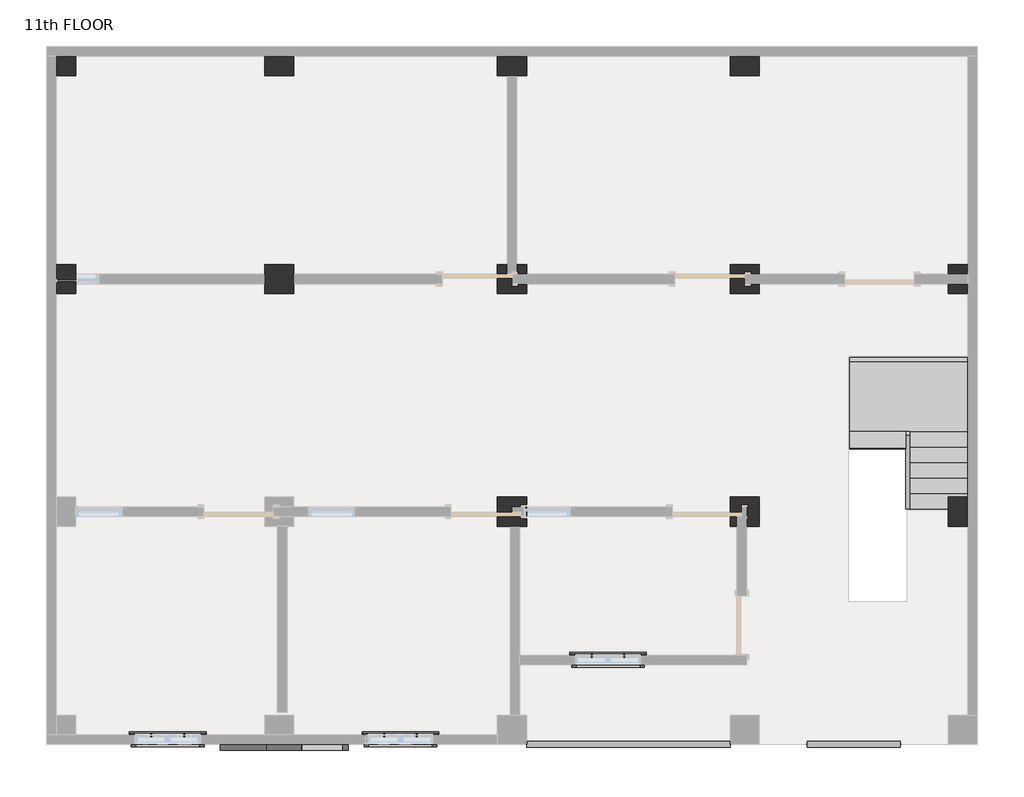
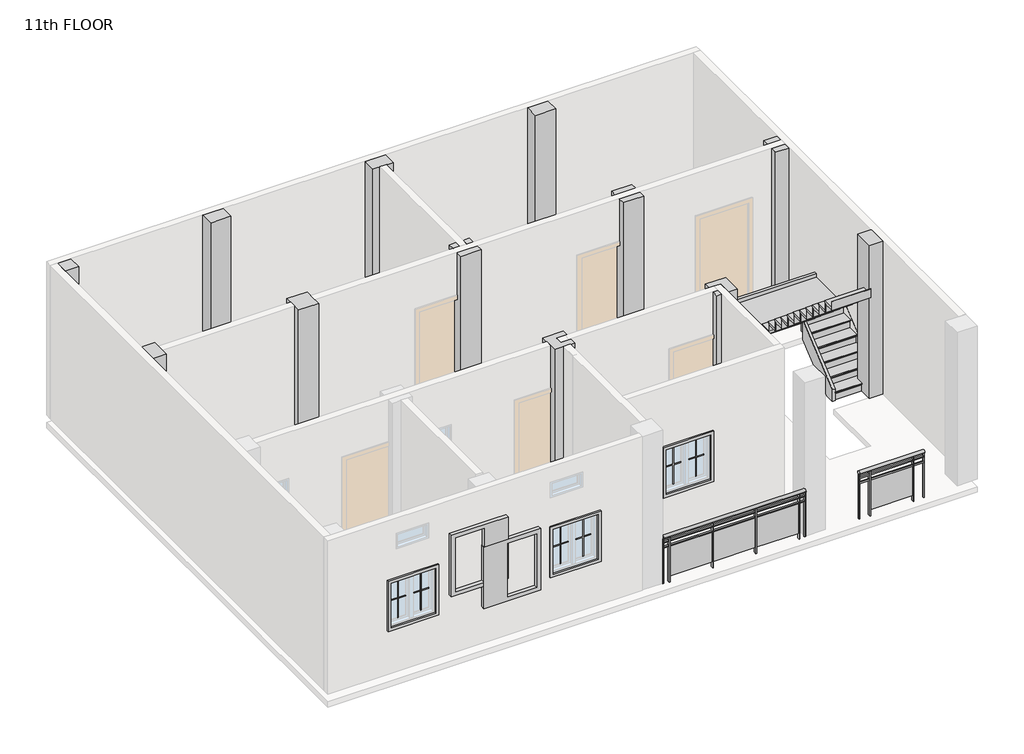
# One storey, part 2 of 2: 12 columns, 12 proxies, 4 members, 2 railings, 1 damper, 1 stair flight.
"""IFC4 building model written with IfcOpenShell, lengths in millimetres."""

from ifc_helpers import new_model, si_unit, point, frame, origin, place, context, project, spatial, polyline, ellipse_curve, trimmed, outline, extrude, faceted_brep, transform, mapped, element, save
from ifc_brep_helpers import plane_surface, extruded_surface, advanced_brep
from components import muntin_pattern_2x2_muntin_pattern_2x2_b3fe6957, muntin_pattern_2x2_muntin_pattern_2x2_3e0ecaf2, trim_window_exterior_flat_with_sill_41619996, trim_window_interior_flat_picture_frame_51c85655, duct_accessories_2_duct_accessories_1_b7e40825, stair_flight_8b765581

model = new_model("IFC4")

# Units and contexts
model_context = context("Model", 3, world=origin())
ifc_project = project(units=[si_unit("LENGTHUNIT", "METRE", prefix="MILLI")], contexts=[model_context])

# Site, building, storey
site = spatial("IfcSite", under=ifc_project)
building = spatial("IfcBuilding", under=site)
storey = spatial("IfcBuildingStorey", under=building, Name="11th FLOOR", Elevation=33375.6)

# Proxies
placement = place(None, origin())
muntin_pattern_2x2_muntin_pattern_2x2_shape = muntin_pattern_2x2_muntin_pattern_2x2_b3fe6957(model_context)
element("IfcBuildingElementProxy", 1, Name="Muntin Pattern_2x2 : Muntin Pattern_2x2", ObjectType="Muntin Pattern_2x2 : Muntin Pattern_2x2", at=placement, inside=storey, context=model_context, shape_type="MappedRepresentation", body=[
    mapped(muntin_pattern_2x2_muntin_pattern_2x2_shape, transform((-14441.409625, -253.8184478, 34359.85), x_axis=(1.0, 0.0, 0.0), y_axis=(0.0, 1.0, 0.0), z_axis=(0.0, 0.0, 1.0))),
])
element("IfcBuildingElementProxy", 2, Name="Muntin Pattern_2x2 : Muntin Pattern_2x2", ObjectType="Muntin Pattern_2x2 : Muntin Pattern_2x2", at=placement, inside=storey, context=model_context, shape_type="MappedRepresentation", body=[
    mapped(muntin_pattern_2x2_muntin_pattern_2x2_shape, transform((-11393.409625, -253.8184478, 34359.85), x_axis=(1.0, 0.0, 0.0), y_axis=(0.0, 1.0, 0.0), z_axis=(0.0, 0.0, 1.0))),
])
element("IfcBuildingElementProxy", 3, Name="Muntin Pattern_2x2 : Muntin Pattern_2x2", ObjectType="Muntin Pattern_2x2 : Muntin Pattern_2x2", at=placement, inside=storey, context=model_context, shape_type="MappedRepresentation", body=[
    mapped(muntin_pattern_2x2_muntin_pattern_2x2_shape, transform((-8675.609625, 787.5815522, 34359.85), x_axis=(1.0, 0.0, 0.0), y_axis=(0.0, 1.0, 0.0), z_axis=(0.0, 0.0, 1.0))),
])
muntin_pattern_2x2_muntin_pattern_2x2_2_shape = muntin_pattern_2x2_muntin_pattern_2x2_3e0ecaf2(model_context)
element("IfcBuildingElementProxy", 4, Name="Muntin Pattern_2x2 : Muntin Pattern_2x2", ObjectType="Muntin Pattern_2x2 : Muntin Pattern_2x2", at=placement, inside=storey, context=model_context, shape_type="MappedRepresentation", body=[
    mapped(muntin_pattern_2x2_muntin_pattern_2x2_2_shape, transform((-14012.784625, -253.8184478, 34359.85), x_axis=(-1.0, 0.0, 0.0), y_axis=(0.0, -1.0, 0.0), z_axis=(0.0, 0.0, 1.0))),
])
element("IfcBuildingElementProxy", 5, Name="Muntin Pattern_2x2 : Muntin Pattern_2x2", ObjectType="Muntin Pattern_2x2 : Muntin Pattern_2x2", at=placement, inside=storey, context=model_context, shape_type="MappedRepresentation", body=[
    mapped(muntin_pattern_2x2_muntin_pattern_2x2_2_shape, transform((-10964.784625, -253.8184478, 34359.85), x_axis=(-1.0, 0.0, 0.0), y_axis=(0.0, -1.0, 0.0), z_axis=(0.0, 0.0, 1.0))),
])
element("IfcBuildingElementProxy", 6, Name="Muntin Pattern_2x2 : Muntin Pattern_2x2", ObjectType="Muntin Pattern_2x2 : Muntin Pattern_2x2", at=placement, inside=storey, context=model_context, shape_type="MappedRepresentation", body=[
    mapped(muntin_pattern_2x2_muntin_pattern_2x2_2_shape, transform((-8246.984625, 787.5815522, 34359.85), x_axis=(-1.0, 0.0, 0.0), y_axis=(0.0, -1.0, 0.0), z_axis=(0.0, 0.0, 1.0))),
])
trim_window_exterior_flat_with_sill_shape = trim_window_exterior_flat_with_sill_41619996(model_context)
element("IfcBuildingElementProxy", 7, Name="Trim-Window-Exterior-Flat : with Sill", ObjectType="Trim-Window-Exterior-Flat : with Sill", at=placement, inside=storey, context=model_context, shape_type="MappedRepresentation", body=[
    mapped(trim_window_exterior_flat_with_sill_shape, transform((-14227.097125, -244.2934478, 35204.4), x_axis=(-1.0, 0.0, 0.0), y_axis=(0.0, 0.0, 1.0), z_axis=(0.0, 1.0, 0.0))),
])
element("IfcBuildingElementProxy", 8, Name="Trim-Window-Exterior-Flat : with Sill", ObjectType="Trim-Window-Exterior-Flat : with Sill", at=placement, inside=storey, context=model_context, shape_type="MappedRepresentation", body=[
    mapped(trim_window_exterior_flat_with_sill_shape, transform((-11179.097125, -244.2934478, 35204.4), x_axis=(-1.0, 0.0, 0.0), y_axis=(0.0, 0.0, 1.0), z_axis=(0.0, 1.0, 0.0))),
])
element("IfcBuildingElementProxy", 9, Name="Trim-Window-Exterior-Flat : with Sill", ObjectType="Trim-Window-Exterior-Flat : with Sill", at=placement, inside=storey, context=model_context, shape_type="MappedRepresentation", body=[
    mapped(trim_window_exterior_flat_with_sill_shape, transform((-8461.297125, 797.1065522, 35204.4), x_axis=(-1.0, 0.0, 0.0), y_axis=(0.0, 0.0, 1.0), z_axis=(0.0, 1.0, 0.0))),
])
trim_window_interior_flat_picture_frame_shape = trim_window_interior_flat_picture_frame_51c85655(model_context)
element("IfcBuildingElementProxy", 10, Name="Trim-Window-Interior-Flat : Picture Frame", ObjectType="Trim-Window-Interior-Flat : Picture Frame", at=placement, inside=storey, context=model_context, shape_type="MappedRepresentation", body=[
    mapped(trim_window_interior_flat_picture_frame_shape, transform((-14227.097125, -371.2934478, 35204.4), x_axis=(1.0, 0.0, 0.0), y_axis=(0.0, 0.0, 1.0), z_axis=(0.0, -1.0, 0.0))),
])
element("IfcBuildingElementProxy", 11, Name="Trim-Window-Interior-Flat : Picture Frame", ObjectType="Trim-Window-Interior-Flat : Picture Frame", at=placement, inside=storey, context=model_context, shape_type="MappedRepresentation", body=[
    mapped(trim_window_interior_flat_picture_frame_shape, transform((-11179.097125, -371.2934478, 35204.4), x_axis=(1.0, 0.0, 0.0), y_axis=(0.0, 0.0, 1.0), z_axis=(0.0, -1.0, 0.0))),
])
element("IfcBuildingElementProxy", 12, Name="Trim-Window-Interior-Flat : Picture Frame", ObjectType="Trim-Window-Interior-Flat : Picture Frame", at=placement, inside=storey, context=model_context, shape_type="MappedRepresentation", body=[
    mapped(trim_window_interior_flat_picture_frame_shape, transform((-8461.297125, 670.1065522, 35204.4), x_axis=(1.0, 0.0, 0.0), y_axis=(0.0, 0.0, 1.0), z_axis=(0.0, -1.0, 0.0))),
])

# Columns
element("IfcColumn", 13, ObjectType="column family : column family", at=placement, inside=storey, context=model_context, shape_type="SweptSolid", body=[
    extrude(outline(polyline([(-15433.597125, 8645.7065522), (-15433.597125, 8391.7065522), (-15687.597125, 8391.7065522), (-15687.597125, 8645.7065522), (-15433.597125, 8645.7065522)])), frame((0.0, 0.0, 33380.6), z_axis=(0.0, 0.0, 1.0), x_axis=(1.0, 0.0, 0.0)), (0.0, 0.0, 1.0), 3038.0),
])
element("IfcColumn", 14, ObjectType="column family : column family", at=placement, inside=storey, context=model_context, shape_type="SweptSolid", body=[
    extrude(outline(polyline([(-12576.097125, 5915.2065522), (-12576.097125, 5534.2065522), (-12957.097125, 5534.2065522), (-12957.097125, 5915.2065522), (-12576.097125, 5915.2065522)])), frame((0.0, 0.0, 33380.6), z_axis=(0.0, 0.0, 1.0), x_axis=(1.0, 0.0, 0.0)), (0.0, 0.0, 1.0), 3038.0),
])
element("IfcColumn", 15, ObjectType="column family : column family", at=placement, inside=storey, context=model_context, shape_type="Brep", body=[
    faceted_brep([(-9655.097125, 5915.2065522, 33380.6), (-9528.097125, 5915.2065522, 33380.6), (-9528.097125, 5788.2065522, 33380.6), (-9655.097125, 5788.2065522, 33380.6), (-9528.097125, 5915.2065522, 36418.6), (-9655.097125, 5915.2065522, 36418.6), (-9655.097125, 5788.2065522, 36418.6), (-9528.097125, 5788.2065522, 36418.6)], [[[0, 1, 2, 3]], [[4, 5, 6, 7]], [[0, 3, 6, 5]], [[4, 1, 0, 5]], [[3, 2, 7, 6]], [[1, 4, 7, 2]]]),
    faceted_brep([(-9528.097125, 5534.2065522, 36418.6), (-9528.097125, 5534.2065522, 33380.6), (-9528.097125, 5661.2065522, 33380.6), (-9528.097125, 5661.2065522, 36418.6), (-9909.097125, 5534.2065522, 33380.6), (-9909.097125, 5534.2065522, 36418.6), (-9909.097125, 5915.2065522, 33380.6), (-9909.097125, 5661.2065522, 36418.6), (-9909.097125, 5661.2065522, 35509.2), (-9909.097125, 5788.2065522, 35509.2), (-9909.097125, 5788.2065522, 36418.6), (-9909.097125, 5915.2065522, 36418.6), (-9782.097125, 5915.2065522, 36418.6), (-9782.097125, 5915.2065522, 33380.6), (-9782.097125, 5788.2065522, 33380.6), (-9782.097125, 5788.2065522, 36418.6), (-9782.097125, 5788.2065522, 35509.2), (-9718.597125, 5788.2065522, 33380.6), (-9718.597125, 5788.2065522, 35509.2), (-9718.597125, 5661.2065522, 33380.6), (-9718.597125, 5661.2065522, 35509.2)], [[[0, 1, 2, 3]], [[4, 1, 0, 5]], [[6, 4, 5, 7, 8, 9, 10, 11]], [[6, 11, 12, 13]], [[14, 13, 12, 15, 16]], [[17, 14, 16, 18]], [[19, 20, 8, 7, 3, 2]], [[1, 4, 6, 13, 14, 17, 19, 2]], [[5, 0, 3, 7]], [[12, 11, 10, 15]], [[9, 16, 15, 10]], [[18, 20, 19, 17]], [[20, 18, 16, 9, 8]]]),
])
element("IfcColumn", 16, ObjectType="column family : column family", at=placement, inside=storey, context=model_context, shape_type="Brep", body=[
    faceted_brep([(-6480.097125, 5534.2065522, 33380.6), (-6861.097125, 5534.2065522, 33380.6), (-6861.097125, 5915.2065522, 33380.6), (-6480.097125, 5915.2065522, 33380.6), (-6480.097125, 5788.2065522, 33380.6), (-6670.597125, 5788.2065522, 33380.6), (-6670.597125, 5661.2065522, 33380.6), (-6480.097125, 5661.2065522, 33380.6), (-6480.097125, 5534.2065522, 36418.6), (-6480.097125, 5661.2065522, 36418.6), (-6861.097125, 5534.2065522, 36418.6), (-6861.097125, 5661.2065522, 36418.6), (-6861.097125, 5661.2065522, 35509.2), (-6861.097125, 5788.2065522, 35509.2), (-6861.097125, 5788.2065522, 36418.6), (-6861.097125, 5915.2065522, 36418.6), (-6480.097125, 5915.2065522, 36418.6), (-6670.597125, 5661.2065522, 35509.2), (-6670.597125, 5788.2065522, 35509.2), (-6480.097125, 5788.2065522, 36418.6)], [[[0, 1, 2, 3, 4, 5, 6, 7]], [[8, 0, 7, 9]], [[1, 0, 8, 10]], [[2, 1, 10, 11, 12, 13, 14, 15]], [[3, 2, 15, 16]], [[10, 8, 9, 11]], [[6, 17, 12, 11, 9, 7]], [[13, 18, 5, 4, 19, 14]], [[3, 16, 19, 4]], [[16, 15, 14, 19]], [[18, 17, 6, 5]], [[17, 18, 13, 12]]]),
])
element("IfcColumn", 17, ObjectType="column family : column family", at=placement, inside=storey, context=model_context, shape_type="Brep", body=[
    faceted_brep([(-6480.097125, 2867.2065522, 33380.6), (-6480.097125, 2486.2065522, 33380.6), (-6645.197125, 2486.2065522, 33380.6), (-6645.197125, 2740.2065522, 33380.6), (-6708.697125, 2740.2065522, 33380.6), (-6708.697125, 2613.2065522, 33380.6), (-6772.197125, 2613.2065522, 33380.6), (-6772.197125, 2486.2065522, 33380.6), (-6861.097125, 2486.2065522, 33380.6), (-6861.097125, 2867.2065522, 33380.6), (-6480.097125, 2867.2065522, 36418.6), (-6480.097125, 2486.2065522, 36418.6), (-6861.097125, 2486.2065522, 36418.6), (-6772.197125, 2486.2065522, 36418.6), (-6861.097125, 2613.2065522, 36418.6), (-6861.097125, 2613.2065522, 35509.2), (-6861.097125, 2740.2065522, 35509.2), (-6861.097125, 2740.2065522, 36418.6), (-6861.097125, 2867.2065522, 36418.6), (-6772.197125, 2740.2065522, 36418.6), (-6645.197125, 2740.2065522, 36418.6), (-6645.197125, 2486.2065522, 36418.6), (-6772.197125, 2613.2065522, 36418.6), (-6772.197125, 2613.2065522, 35509.2), (-6772.197125, 2740.2065522, 35509.2), (-6708.697125, 2613.2065522, 35509.2), (-6708.697125, 2740.2065522, 35509.2)], [[[0, 1, 2, 3, 4, 5, 6, 7, 8, 9]], [[1, 0, 10, 11]], [[12, 8, 7, 13]], [[9, 8, 12, 14, 15, 16, 17, 18]], [[0, 9, 18, 10]], [[11, 10, 18, 17, 19, 20, 21]], [[15, 14, 22, 23]], [[17, 16, 24, 19]], [[20, 3, 2, 21]], [[6, 23, 22, 13, 7]], [[14, 12, 13, 22]], [[1, 11, 21, 2]], [[15, 23, 24, 16]], [[25, 23, 6, 5]], [[23, 25, 26, 24]], [[26, 25, 5, 4]], [[24, 26, 4, 3, 20, 19]]]),
])
element("IfcColumn", 18, ObjectType="column family : column family", at=placement, inside=storey, context=model_context, shape_type="Brep", body=[
    faceted_brep([(-9528.097125, 2486.2065522, 33380.6), (-9909.097125, 2486.2065522, 33380.6), (-9909.097125, 2867.2065522, 33380.6), (-9528.097125, 2867.2065522, 33380.6), (-9528.097125, 2740.2065522, 33380.6), (-9566.197125, 2740.2065522, 33380.6), (-9718.597125, 2740.2065522, 33380.6), (-9718.597125, 2613.2065522, 33380.6), (-9566.197125, 2613.2065522, 33380.6), (-9528.097125, 2613.2065522, 33380.6), (-9528.097125, 2486.2065522, 36418.6), (-9528.097125, 2613.2065522, 33680.4), (-9528.097125, 2740.2065522, 33680.4), (-9528.097125, 2867.2065522, 36418.6), (-9528.097125, 2740.2065522, 36418.6), (-9528.097125, 2740.2065522, 35509.2), (-9528.097125, 2613.2065522, 35509.2), (-9528.097125, 2613.2065522, 36418.6), (-9909.097125, 2486.2065522, 36418.6), (-9909.097125, 2867.2065522, 36418.6), (-9566.197125, 2613.2065522, 36418.6), (-9718.597125, 2613.2065522, 36418.6), (-9718.597125, 2740.2065522, 36418.6), (-9566.197125, 2740.2065522, 36418.6), (-9566.197125, 2613.2065522, 35509.2), (-9566.197125, 2613.2065522, 33680.4), (-9566.197125, 2740.2065522, 33680.4), (-9566.197125, 2740.2065522, 35509.2)], [[[0, 1, 2, 3, 4, 5, 6, 7, 8, 9]], [[10, 0, 9, 11, 12, 4, 3, 13, 14, 15, 16, 17]], [[1, 0, 10, 18]], [[2, 1, 18, 19]], [[3, 2, 19, 13]], [[18, 10, 17, 20, 21, 22, 23, 14, 13, 19]], [[11, 9, 8, 7, 21, 20, 17, 16, 24, 25]], [[4, 12, 26, 27, 15, 14, 23, 22, 6, 5]], [[21, 7, 6, 22]], [[25, 24, 27, 26]], [[25, 26, 12, 11]], [[27, 24, 16, 15]]]),
])
element("IfcColumn", 19, ObjectType="column family : column family", at=placement, inside=storey, context=model_context, shape_type="SweptSolid", body=[
    extrude(outline(polyline([(-12576.097125, 8391.7065522), (-12957.097125, 8391.7065522), (-12957.097125, 8645.7065522), (-12576.097125, 8645.7065522), (-12576.097125, 8391.7065522)])), frame((0.0, 0.0, 33380.6), z_axis=(0.0, 0.0, 1.0), x_axis=(1.0, 0.0, 0.0)), (0.0, 0.0, 1.0), 3038.0),
])
element("IfcColumn", 20, ObjectType="column family : column family", at=placement, inside=storey, context=model_context, shape_type="SweptSolid", body=[
    extrude(outline(polyline([(-9528.097125, 8391.7065522), (-9909.097125, 8391.7065522), (-9909.097125, 8645.7065522), (-9528.097125, 8645.7065522), (-9528.097125, 8391.7065522)])), frame((0.0, 0.0, 33380.6), z_axis=(0.0, 0.0, 1.0), x_axis=(1.0, 0.0, 0.0)), (0.0, 0.0, 1.0), 3038.0),
])
element("IfcColumn", 21, ObjectType="column family : column family", at=placement, inside=storey, context=model_context, shape_type="SweptSolid", body=[
    extrude(outline(polyline([(-6480.097125, 8391.7065522), (-6861.097125, 8391.7065522), (-6861.097125, 8645.7065522), (-6480.097125, 8645.7065522), (-6480.097125, 8391.7065522)])), frame((0.0, 0.0, 33380.6), z_axis=(0.0, 0.0, 1.0), x_axis=(1.0, 0.0, 0.0)), (0.0, 0.0, 1.0), 3038.0),
])
element("IfcColumn", 22, ObjectType="column family : column family", at=placement, inside=storey, context=model_context, shape_type="SweptSolid", body=[
    extrude(outline(polyline([(-4003.597125, 5915.2065522), (-3749.597125, 5915.2065522), (-3749.597125, 5788.2065522), (-4003.597125, 5788.2065522), (-4003.597125, 5915.2065522)])), frame((0.0, 0.0, 33380.6), z_axis=(0.0, 0.0, 1.0), x_axis=(1.0, 0.0, 0.0)), (0.0, 0.0, 1.0), 3038.0),
    extrude(outline(polyline([(-3749.597125, 5534.2065522), (-4003.597125, 5534.2065522), (-4003.597125, 5661.2065522), (-3749.597125, 5661.2065522), (-3749.597125, 5534.2065522)])), frame((0.0, 0.0, 33380.6), z_axis=(0.0, 0.0, 1.0), x_axis=(1.0, 0.0, 0.0)), (0.0, 0.0, 1.0), 3038.0),
])
element("IfcColumn", 23, ObjectType="column family : column family", at=placement, inside=storey, context=model_context, shape_type="SweptSolid", body=[
    extrude(outline(polyline([(-4003.597125, 2486.2065522), (-4003.597125, 2867.2065522), (-3749.597125, 2867.2065522), (-3749.597125, 2486.2065522), (-4003.597125, 2486.2065522)])), frame((0.0, 0.0, 33380.6), z_axis=(0.0, 0.0, 1.0), x_axis=(1.0, 0.0, 0.0)), (0.0, 0.0, 1.0), 3038.0),
])
element("IfcColumn", 24, ObjectType="column family : column family", at=placement, inside=storey, context=model_context, shape_type="SweptSolid", body=[
    extrude(outline(polyline([(-15433.597125, 5915.2065522), (-15433.597125, 5534.2065522), (-15687.597125, 5534.2065522), (-15687.597125, 5915.2065522), (-15433.597125, 5915.2065522)])), frame((0.0, 0.0, 33380.6), z_axis=(0.0, 0.0, 1.0), x_axis=(1.0, 0.0, 0.0)), (0.0, 0.0, 1.0), 3038.0),
])

# Damper
duct_accessories_2_duct_accessories_1_shape = duct_accessories_2_duct_accessories_1_b7e40825(model_context)
element("IfcDamper", 25, ObjectType="Duct Accessories 2 : Duct Accessories 1", at=placement, inside=storey, context=model_context, shape_type="MappedRepresentation", body=[
    mapped(duct_accessories_2_duct_accessories_1_shape, transform((0.0, 0.0, 0.0), x_axis=(1.0, 0.0, 0.0), y_axis=(0.0, 1.0, 0.0), z_axis=(0.0, 0.0, 1.0))),
])

# Members
element("IfcMember", 26, ObjectType="Stringer - 2\" Width", at=placement, inside=storey, context=model_context, shape_type="SweptSolid", body=[
    extrude(outline(polyline([(2714.6319226, 33375.6), (2714.6319226, 33612.4438745), (3679.8319226, 34416.7772078), (3679.8319226, 34020.0165243), (2906.5320935, 33375.6), (2714.6319226, 33375.6)])), frame((-4563.0136682, 0.0, 0.0), z_axis=(1.0, 0.0, 0.0), x_axis=(0.0, 1.0, 0.0)), (0.0, 0.0, 1.0), 50.8),
])
element("IfcMember", 27, ObjectType="Stringer - 2\" Width", at=placement, inside=storey, context=model_context, shape_type="SweptSolid", body=[
    extrude(outline(polyline([(-4512.2136682, 3730.6319226), (-4512.2136682, 3679.8319226), (-4563.0136682, 3679.8319226), (-4563.0136682, 3730.6319226), (-4512.2136682, 3730.6319226)])), frame((0.0, 0.0, 34163.0), z_axis=(0.0, 0.0, 1.0), x_axis=(1.0, 0.0, 0.0)), (0.0, 0.0, 1.0), 304.8),
])
element("IfcMember", 28, ObjectType="Stringer - 2\" Width", at=placement, inside=storey, context=model_context, shape_type="SweptSolid", body=[
    extrude(outline(polyline([(2714.6319226, 33375.6), (2714.6319226, 33612.4438745), (3741.0592732, 34467.8), (4217.1720935, 34467.8), (2906.5320935, 33375.6), (2714.6319226, 33375.6)])), frame((-3749.597125, 0.0, 0.0), z_axis=(1.0, 0.0, 0.0), x_axis=(0.0, 1.0, 0.0)), (0.0, 0.0, 1.0), 50.8),
])
element("IfcMember", 29, ObjectType="Stringer - 2\" Width", at=placement, inside=storey, context=model_context, shape_type="SweptSolid", body=[
    extrude(outline(polyline([(-3698.797125, 4695.8319226), (-3698.797125, 4645.0319226), (-5295.0246464, 4645.0319226), (-5295.0246464, 4695.8319226), (-3698.797125, 4695.8319226)])), frame((0.0, 0.0, 34163.0), z_axis=(0.0, 0.0, 1.0), x_axis=(1.0, 0.0, 0.0)), (0.0, 0.0, 1.0), 304.8),
])

# Railings
element("IfcRailing", 30, ObjectType="Glass Panel - Bottom Fill", at=placement, inside=storey, context=model_context, shape_type="SolidModel", body=[
    advanced_brep(
    [(-9528.097125, -333.1934478, 34290.0), (-9528.097125, -409.3934478, 34290.0), (-6861.097125, -333.1934478, 34290.0), (-6861.097125, -409.3934478, 34290.0)],
    [
        (0, 1, ellipse_curve(frame((-9528.097125, -371.2934478, 34290.0), z_axis=(-1.0, 0.0, 0.0), x_axis=(0.0, -1.0, 0.0)), 38.1, 28.575)),
        (1, 0, ellipse_curve(frame((-9528.097125, -371.2934478, 34290.0), z_axis=(-1.0, 0.0, 0.0), x_axis=(0.0, -1.0, 0.0)), 38.1, 28.575)),
        (2, 3, ellipse_curve(frame((-6861.097125, -371.2934478, 34290.0), z_axis=(1.0, 0.0, 0.0), x_axis=(0.0, -1.0, 0.0)), 38.1, 28.575)),
        (3, 2, ellipse_curve(frame((-6861.097125, -371.2934478, 34290.0), z_axis=(1.0, 0.0, 0.0), x_axis=(0.0, -1.0, 0.0)), 38.1, 28.575)),
        (0, 2),
        (3, 1),
    ],
    [
        plane_surface(frame((-9528.097125, -371.2934478, 34290.0), z_axis=(-1.0, 0.0, 0.0), x_axis=(0.0, 1.0, 0.0))),
        plane_surface(frame((-6861.097125, -371.2934478, 34290.0), z_axis=(1.0, 0.0, 0.0), x_axis=(0.0, 1.0, 0.0))),
        extruded_surface(trimmed(ellipse_curve(frame((-6861.097125, -371.2934478, 34290.0), z_axis=(-1.0, 0.0, 0.0), x_axis=(0.0, -1.0, 0.0)), 38.1, 28.575), [point((-6861.097125, -333.1934478, 34290.0))], [point((-6861.097125, -409.3934478, 34290.0))], True, "CARTESIAN"), (-2667.0, 0.0, 0.0), 2667.0),
        extruded_surface(trimmed(ellipse_curve(frame((-6861.097125, -371.2934478, 34290.0), z_axis=(-1.0, 0.0, 0.0), x_axis=(0.0, -1.0, 0.0)), 38.1, 28.575), [point((-6861.097125, -409.3934478, 34290.0))], [point((-6861.097125, -333.1934478, 34290.0))], True, "CARTESIAN"), (-2667.0, 0.0, 0.0), 2667.0),
    ],
    [
        (0, [[1, 2]]),
        (1, [[3, 4]]),
        (2, [[-1, 5, -4, 6]]),
        (3, [[-2, -6, -3, -5]]),
    ],
),
    extrude(outline(polyline([(-9528.097125, -383.9934478), (-9528.097125, -358.5934478), (-6861.097125, -358.5934478), (-6861.097125, -383.9934478), (-9528.097125, -383.9934478)])), frame((0.0, 0.0, 34175.7), z_axis=(0.0, 0.0, 1.0), x_axis=(1.0, 0.0, 0.0)), (0.0, 0.0, 1.0), 25.4),
    extrude(outline(polyline([(-9528.097125, -383.9934478), (-9528.097125, -358.5934478), (-6861.097125, -358.5934478), (-6861.097125, -383.9934478), (-9528.097125, -383.9934478)])), frame((0.0, 0.0, 34074.1), z_axis=(0.0, 0.0, 1.0), x_axis=(1.0, 0.0, 0.0)), (0.0, 0.0, 1.0), 25.4),
    extrude(outline(polyline([(-6981.747125, -396.6934478), (-6981.747125, -345.8934478), (-6969.047125, -345.8934478), (-6969.047125, -396.6934478), (-6981.747125, -396.6934478)])), frame((0.0, 0.0, 33375.6), z_axis=(0.0, 0.0, 1.0), x_axis=(1.0, 0.0, 0.0)), (0.0, 0.0, 1.0), 885.6788223),
    extrude(outline(polyline([(-7788.197125, -364.7582908), (-6975.397125, -364.7582908), (-6975.397125, -371.1082908), (-7788.197125, -371.1082908), (-7788.197125, -364.7582908)])), frame((0.0, 0.0, 33477.2), z_axis=(0.0, 0.0, 1.0), x_axis=(1.0, 0.0, 0.0)), (0.0, 0.0, 1.0), 596.9),
    extrude(outline(polyline([(-7794.547125, -396.6934478), (-7794.547125, -345.8934478), (-7781.847125, -345.8934478), (-7781.847125, -396.6934478), (-7794.547125, -396.6934478)])), frame((0.0, 0.0, 33375.6), z_axis=(0.0, 0.0, 1.0), x_axis=(1.0, 0.0, 0.0)), (0.0, 0.0, 1.0), 885.6788223),
    extrude(outline(polyline([(-8600.997125, -364.7582908), (-7788.197125, -364.7582908), (-7788.197125, -371.1082908), (-8600.997125, -371.1082908), (-8600.997125, -364.7582908)])), frame((0.0, 0.0, 33477.2), z_axis=(0.0, 0.0, 1.0), x_axis=(1.0, 0.0, 0.0)), (0.0, 0.0, 1.0), 596.9),
    extrude(outline(polyline([(-8607.347125, -396.6934478), (-8607.347125, -345.8934478), (-8594.647125, -345.8934478), (-8594.647125, -396.6934478), (-8607.347125, -396.6934478)])), frame((0.0, 0.0, 33375.6), z_axis=(0.0, 0.0, 1.0), x_axis=(1.0, 0.0, 0.0)), (0.0, 0.0, 1.0), 885.6788223),
    extrude(outline(polyline([(-9413.797125, -364.7582908), (-8600.997125, -364.7582908), (-8600.997125, -371.1082908), (-9413.797125, -371.1082908), (-9413.797125, -364.7582908)])), frame((0.0, 0.0, 33477.2), z_axis=(0.0, 0.0, 1.0), x_axis=(1.0, 0.0, 0.0)), (0.0, 0.0, 1.0), 596.9),
    extrude(outline(polyline([(-9420.147125, -396.6934478), (-9420.147125, -345.8934478), (-9407.447125, -345.8934478), (-9407.447125, -396.6934478), (-9420.147125, -396.6934478)])), frame((0.0, 0.0, 33375.6), z_axis=(0.0, 0.0, 1.0), x_axis=(1.0, 0.0, 0.0)), (0.0, 0.0, 1.0), 885.6788223),
    extrude(outline(polyline([(-6873.797125, -380.8184478), (-6873.797125, -361.7684478), (-6854.747125, -361.7684478), (-6854.747125, -380.8184478), (-6873.797125, -380.8184478)])), frame((0.0, 0.0, 33375.6), z_axis=(0.0, 0.0, 1.0), x_axis=(1.0, 0.0, 0.0)), (0.0, 0.0, 1.0), 885.6788223),
    extrude(outline(polyline([(-9534.447125, -380.8184478), (-9534.447125, -361.7684478), (-9515.397125, -361.7684478), (-9515.397125, -380.8184478), (-9534.447125, -380.8184478)])), frame((0.0, 0.0, 33375.6), z_axis=(0.0, 0.0, 1.0), x_axis=(1.0, 0.0, 0.0)), (0.0, 0.0, 1.0), 885.6788223),
])
element("IfcRailing", 31, ObjectType="Glass Panel - Bottom Fill", at=placement, inside=storey, context=model_context, shape_type="SolidModel", body=[
    advanced_brep(
    [(-5851.447125, -333.1934478, 34290.0), (-5851.447125, -409.3934478, 34290.0), (-4632.247125, -333.1934478, 34290.0), (-4632.247125, -409.3934478, 34290.0)],
    [
        (0, 1, ellipse_curve(frame((-5851.447125, -371.2934478, 34290.0), z_axis=(-1.0, 0.0, 0.0), x_axis=(0.0, -1.0, 0.0)), 38.1, 28.575)),
        (1, 0, ellipse_curve(frame((-5851.447125, -371.2934478, 34290.0), z_axis=(-1.0, 0.0, 0.0), x_axis=(0.0, -1.0, 0.0)), 38.1, 28.575)),
        (2, 3, ellipse_curve(frame((-4632.247125, -371.2934478, 34290.0), z_axis=(1.0, 0.0, 0.0), x_axis=(0.0, -1.0, 0.0)), 38.1, 28.575)),
        (3, 2, ellipse_curve(frame((-4632.247125, -371.2934478, 34290.0), z_axis=(1.0, 0.0, 0.0), x_axis=(0.0, -1.0, 0.0)), 38.1, 28.575)),
        (0, 2),
        (3, 1),
    ],
    [
        plane_surface(frame((-5851.447125, -371.2934478, 34290.0), z_axis=(-1.0, 0.0, 0.0), x_axis=(0.0, 1.0, 0.0))),
        plane_surface(frame((-4632.247125, -371.2934478, 34290.0), z_axis=(1.0, 0.0, 0.0), x_axis=(0.0, 1.0, 0.0))),
        extruded_surface(trimmed(ellipse_curve(frame((-4632.247125, -371.2934478, 34290.0), z_axis=(-1.0, 0.0, 0.0), x_axis=(0.0, -1.0, 0.0)), 38.1, 28.575), [point((-4632.247125, -333.1934478, 34290.0))], [point((-4632.247125, -409.3934478, 34290.0))], True, "CARTESIAN"), (-1219.1999999999998, 0.0, 0.0), 1219.1999999999998),
        extruded_surface(trimmed(ellipse_curve(frame((-4632.247125, -371.2934478, 34290.0), z_axis=(-1.0, 0.0, 0.0), x_axis=(0.0, -1.0, 0.0)), 38.1, 28.575), [point((-4632.247125, -409.3934478, 34290.0))], [point((-4632.247125, -333.1934478, 34290.0))], True, "CARTESIAN"), (-1219.1999999999998, 0.0, 0.0), 1219.1999999999998),
    ],
    [
        (0, [[1, 2]]),
        (1, [[3, 4]]),
        (2, [[-1, 5, -4, 6]]),
        (3, [[-2, -6, -3, -5]]),
    ],
),
    extrude(outline(polyline([(-5851.447125, -383.9934478), (-5851.447125, -358.5934478), (-4632.247125, -358.5934478), (-4632.247125, -383.9934478), (-5851.447125, -383.9934478)])), frame((0.0, 0.0, 34175.7), z_axis=(0.0, 0.0, 1.0), x_axis=(1.0, 0.0, 0.0)), (0.0, 0.0, 1.0), 25.4),
    extrude(outline(polyline([(-5851.447125, -383.9934478), (-5851.447125, -358.5934478), (-4632.247125, -358.5934478), (-4632.247125, -383.9934478), (-5851.447125, -383.9934478)])), frame((0.0, 0.0, 34074.1), z_axis=(0.0, 0.0, 1.0), x_axis=(1.0, 0.0, 0.0)), (0.0, 0.0, 1.0), 25.4),
    extrude(outline(polyline([(-4841.797125, -396.6934478), (-4841.797125, -345.8934478), (-4829.097125, -345.8934478), (-4829.097125, -396.6934478), (-4841.797125, -396.6934478)])), frame((0.0, 0.0, 33375.6), z_axis=(0.0, 0.0, 1.0), x_axis=(1.0, 0.0, 0.0)), (0.0, 0.0, 1.0), 885.6788223),
    extrude(outline(polyline([(-5648.247125, -364.7582908), (-4835.447125, -364.7582908), (-4835.447125, -371.1082908), (-5648.247125, -371.1082908), (-5648.247125, -364.7582908)])), frame((0.0, 0.0, 33477.2), z_axis=(0.0, 0.0, 1.0), x_axis=(1.0, 0.0, 0.0)), (0.0, 0.0, 1.0), 596.9),
    extrude(outline(polyline([(-5654.597125, -396.6934478), (-5654.597125, -345.8934478), (-5641.897125, -345.8934478), (-5641.897125, -396.6934478), (-5654.597125, -396.6934478)])), frame((0.0, 0.0, 33375.6), z_axis=(0.0, 0.0, 1.0), x_axis=(1.0, 0.0, 0.0)), (0.0, 0.0, 1.0), 885.6788223),
    extrude(outline(polyline([(-4644.947125, -380.8184478), (-4644.947125, -361.7684478), (-4625.897125, -361.7684478), (-4625.897125, -380.8184478), (-4644.947125, -380.8184478)])), frame((0.0, 0.0, 33375.6), z_axis=(0.0, 0.0, 1.0), x_axis=(1.0, 0.0, 0.0)), (0.0, 0.0, 1.0), 885.6788223),
    extrude(outline(polyline([(-5857.797125, -380.8184478), (-5857.797125, -361.7684478), (-5838.747125, -361.7684478), (-5838.747125, -380.8184478), (-5857.797125, -380.8184478)])), frame((0.0, 0.0, 33375.6), z_axis=(0.0, 0.0, 1.0), x_axis=(1.0, 0.0, 0.0)), (0.0, 0.0, 1.0), 885.6788223),
])

# Stair flight
stair_flight_shape = stair_flight_8b765581(model_context)
element("IfcStairFlight", 32, ObjectType="2\" Tread 1\" Nosing 1/4\" Riser", at=placement, inside=storey, context=model_context, shape_type="MappedRepresentation", body=[
    mapped(stair_flight_shape, transform((0.0, 0.0, 0.0), x_axis=(1.0, 0.0, 0.0), y_axis=(0.0, 1.0, 0.0), z_axis=(0.0, 0.0, 1.0))),
])

save(model, "model.ifc")

# Revit data of these elements
# Type "Muntin Pattern_2x2 : Muntin Pattern_2x2"
#   Width [instance default] = 4' - 0"
#   Thickness = 0' - 0 1/2"
#   Height [instance default] = 4' - 0"
#   Distance = 0' - 0 3/4"
#   Interior Material [instance default] = none
#   Exterior Material [instance default] = none
#   Default Elevation = 0
# Type "Trim-Window-Exterior-Flat : with Sill"
#   Trim Width = 0' - 2 1/4"
#   Trim Thickness_Picture Frame = 0' - 1 1/4"
#   Trim Thickness_with Sill = 0' - 0 3/4"
#   Sill Thickness = 0' - 1 1/4"
#   Opening Width [instance default] = 2' - 0"
#   Opening Height [instance default] = 3' - 0"
#   Default Elevation = 4' - 0"
#   Sill = yes
#   Picture Frame = no
#   Trim Material [instance default] = none
# Type "Trim-Window-Interior-Flat : Picture Frame"
#   Trim Thickness_Picture Frame = 0' - 1 1/4"
#   Trim Width = 0' - 2 1/4"
#   Trim Thickness_with Sill = 0' - 0 3/4"
#   Sill Thickness = 0' - 1 1/4"
#   Opening Width [instance default] = 2' - 0"
#   Opening Height [instance default] = 3' - 0"
#   Default Elevation = 4' - 0"
#   Sill = no
#   Picture Frame = yes
#   Trim Material [instance default] = none
# Type "column family : column family"
#   w2 [instance default] = 0' - 9.88189"
#   w1 [instance default] = 0' - 9.01575"
#   Depth = 1' - 11.62205"
#   Width = 1' - 11.62205"
# Type "Glass Panel - Bottom Fill"
#   Assembly Code = "C2010400"
#   built-in parameter 1008612 = 0.0416667 (stored number, unit not read)
#   built-in parameter 1008611 = 0.0416667 (stored number, unit not read)
#   built-in parameter 1008609 = 0.333333 (stored number, unit not read)
#   built-in parameter 1008604 = 0.166667 (stored number, unit not read)
#   built-in parameter 1008603 = 0.166667 (stored number, unit not read)
#   Railing Height = 3' - 0"
#   built-in parameter 1008630 = 2
#   built-in parameter 1008610 = 2
#   built-in parameter 1008618 = Baluster - Square : 3/4"
# Elements 1, 2, 3, 4, 5, 6 (IfcBuildingElementProxy, "Muntin Pattern_2x2 : Muntin Pattern_2x2")
#   Width = 0' - 11 5/8"
#   Height = 2' - 6 1/2"
#   Interior Material = Wood - Stained
#   Exterior Material = Clad - White
#   Phase Created = New Construction
#   Materials on its faces: "Clad - White", "Wood - Stained"
# Elements 7, 8, 9 (IfcBuildingElementProxy, "Trim-Window-Exterior-Flat : with Sill")
#   Opening Width = 2' - 10"
#   Opening Height = 3' - 0"
#   Trim Material = Clad - White
#   Phase Created = New Construction
#   Materials on its faces: "Clad - White"
# Elements 10, 11, 12 (IfcBuildingElementProxy, "Trim-Window-Interior-Flat : Picture Frame")
#   Opening Width = 2' - 10"
#   Opening Height = 3' - 0"
#   Trim Material = Wood - Stained
#   Phase Created = New Construction
#   Materials on its faces: "Wood - Stained"
# Elements 13, 14, 15, 19, 20, 21 (IfcColumn, "column family : column family")
#   w2 = 1' - 3"
#   w1 = 1' - 3"
#   Phase Created = New Construction
#   Materials on its faces: "Default Wall"
# Elements 16, 22, 23 (IfcColumn, "column family : column family")
#   w2 = 1' - 3"
#   w1 = 1' - 3"
#   Phase Created = New Construction
#   Materials on its faces: "grey", "Default Wall"
# Elements 17, 18 (IfcColumn, "column family : column family")
#   w2 = 1' - 3"
#   w1 = 1' - 3"
#   Phase Created = New Construction
#   Materials on its faces: "Default Wall", "inside wall"
# Element 24 (IfcColumn, "column family : column family")
#   w2 = 1' - 3"
#   w1 = 1' - 3"
#   Phase Created = New Construction
#   Materials on its faces: "inside wall", "Default Wall"
# Element 25 (IfcDamper, "Duct Accessories 2 : Duct Accessories 1")
#   Mark = "2"
#   Phase Created = New Construction
#   Materials on its faces: "border"
# Elements 26, 27, 28, 29 (IfcMember, "Stringer - 2\" Width")
#   Phase Created = New Construction
# Elements 30, 31 (IfcRailing, "Glass Panel - Bottom Fill")
#   Phase Created = New Construction
#   Materials on its faces: "Glass"
# Element 32 (IfcStairFlight, "2\" Tread 1\" Nosing 1/4\" Riser")
#   Phase Created = New Construction
# Materials
#   "Clad - White": class "Wood", colour RGB 242 242 238, transparency 0, Cost = 0
#   "Wood - Stained": class "Wood", colour RGB 224 178 126, transparency 0, Cost = 0
#   "Default Wall": colour RGB 128 128 128, transparency 0, Cost = 0
#   "grey": class "Generic", colour RGB 80 80 80, transparency 0, Cost = 0
#   "inside wall": class "Generic", colour RGB 199 224 95, transparency 0, Cost = 0
#   "border": class "Generic", colour RGB 144 144 144, transparency 0, Cost = 0
#   "Glass": class "Glass", colour RGB 0 128 192, transparency 0.75, Description = "Soda Lime Glass", Cost = 0
